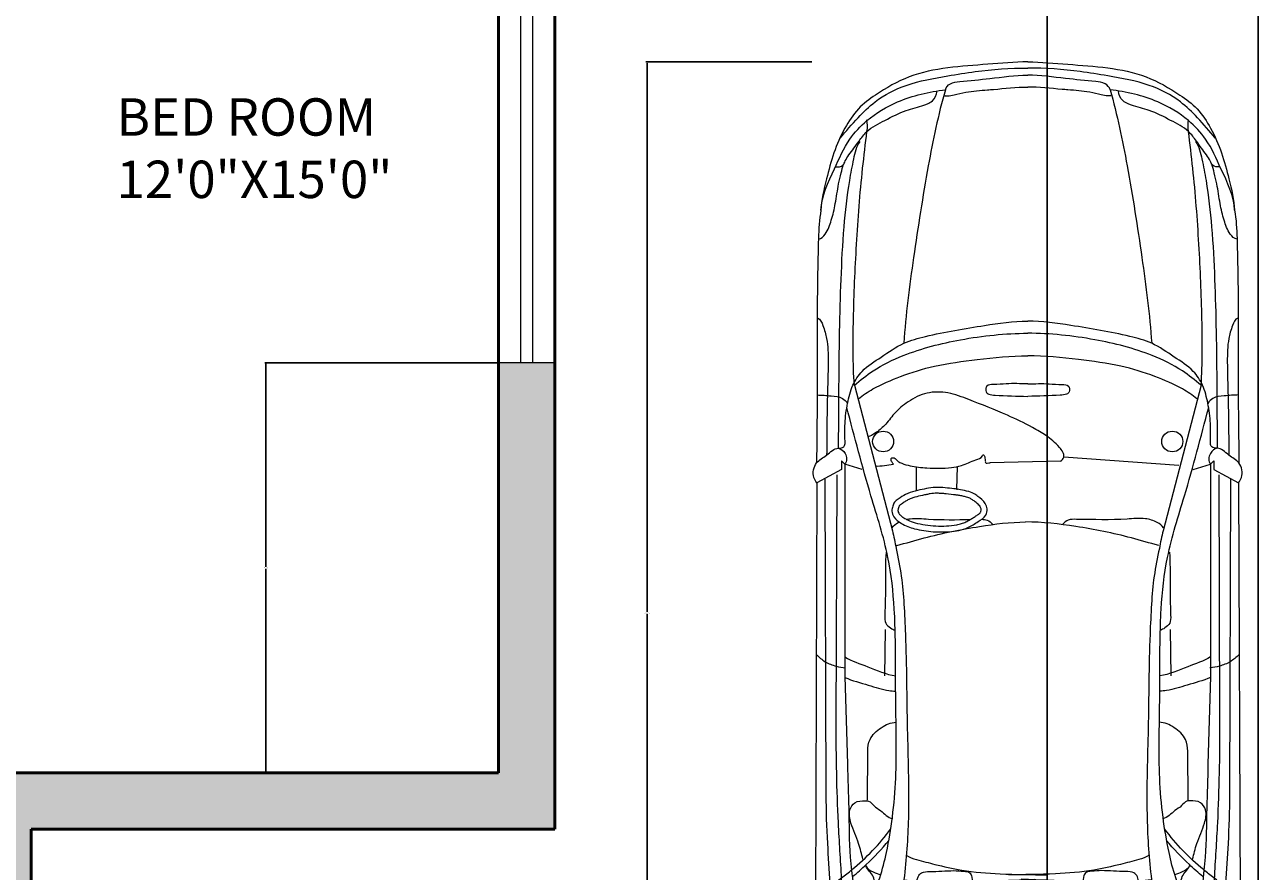
# Model space of a CAD drawing. Units: inches. Extents: x 383 to 970, y 275 to 1088.
# Tile 3 of 11: x 650 to 849, y 410 to 546. Entities that reach past the tile are written whole.
import ezdxf

# ---------------------------------------------------------------- set-up
doc = ezdxf.new("R2010")
doc.units = ezdxf.units.IN
doc.header["$MEASUREMENT"] = 0
for name, color, linetype, lineweight in [('A-ANNO-DIMS', 2, 'Continuous', 18), ('A-AREA-IDEN', 7, 'Continuous', 18), ('A-EQPM-VEHI', 8, 'Continuous', 13), ('A-GLAZ', 4, 'Continuous', 18), ('A-WALL', 7, 'Continuous', 50)]:
    doc.layers.add(name, color=color, linetype=linetype, lineweight=lineweight)
doc.layers.add('A-WALL-PATT', color=251, linetype='Continuous', lineweight=13, true_color=0x636466)
doc.styles.get("Standard").update_dxf_attribs({"font": 'arial.ttf'})
doc.dimstyles.get("Standard").update_dxf_attribs({"dimtxt": 0.18, "dimasz": 0.18, "dimexe": 0.18, "dimexo": 0.0625, "dimgap": 0.09, "dimtad": 0, "dimtih": 1, "dimtoh": 1, "dimdec": 4, "dimzin": 0, "dimdsep": 46, "dimtxsty": 'Standard', "dimcen": 0.09, "dimadec": 0, "dimazin": 0, "dimtfac": 1, "dimtdec": 4, "dimtofl": 0, "dimtmove": 0, "dimatfit": 3, "dimfxl": 1, "dimtolj": 1, "dimtzin": 0, "dimarcsym": 0})

# ---------------------------------------------------------------- blocks, each defined once
blk = doc.blocks.new('A$C242571DA')
for p, q in [((1659.9, 1632), (1714.3, 1732.5)), ((1714.3, 1732.5), (3817.1, 1739.9)), ((1699.9, 1699.4), (2984.7, 1695.8)), ((1638.3, 1618.5), (1625.1, 1632)), ((1625.1, 1632), (1659.9, 1632)), ((1638.3, 1618.5), (2503.3, 1618.5)), ((1659.9, 1548.1), (1638.3, 1618.5)), ((1681.8, 1651.6), (2695.2, 1655.3)), ((2503.3, 1618.5), (2861.6, 1607.5)), ((1317.4, 1579.7), (1909.8, 1424.9)), ((3007.2, 1526.5), (2808.1, 1525.2)), ((1644, 1489.1), (1610.4, 1020.2)), ((2311.9, 1454.3), (2500.6, 1456.9)), ((3474.6, 1401.1), (3474.6, 843)), ((4315.2, 1398), (4377.3, 1370.5)), ((1626.1, 1006.5), (1632.8, 719.7)), ((3474.6, 345.6), (3474.6, 903.8)), ((1740.2, 584.9), (1649.3, 586.9)), ((1746.1, 420.6), (1649.3, 420.6)), ((4315.2, 348.7), (4377.3, 376.3)), ((1317.4, 167), (1909.8, 321.9)), ((2311.9, 292.5), (2500.6, 289.8)), ((3007.2, 220.3), (2808.1, 221.6)), ((1659.9, 198.7), (1638.3, 128.2)), ((1638.3, 128.2), (1625.1, 114.7)), ((1625.1, 114.7), (1659.9, 114.7)), ((1638.3, 128.2), (2503.3, 128.2)), ((1659.9, 114.7), (1714.3, 14.2)), ((2503.3, 128.2), (2861.6, 139.2)), ((1681.8, 95.1), (2695.2, 91.4)), ((1699.9, 47.3), (2984.7, 51)), ((1714.3, 14.2), (3817.1, 6.9))]:
    blk.add_line(p, q)
for centre in [(1546.4, 1462.5), (1546.4, 284.2)]:
    blk.add_ellipse(centre, major_axis=(0, 42.9), ratio=0.983266, start_param=4.712389, end_param=10.995574)
for points, knots in [([(722.7, 1726.6), (720.8, 1714.9), (694.5, 1689.9), (643, 1671.8), (573.6, 1655.4), (508.5, 1647), (455.2, 1634.7), (428.7, 1627.3), (416.9, 1624.1)], [0, 0, 0, 0, 0.034703, 0.0959761, 0.1659336, 0.2471559, 0.2929944, 0.3295918, 0.3295918, 0.3295918, 0.3295918]), ([(604.6, 1715.7), (642.1, 1723.4), (788.5, 1729.2), (1039.3, 1732.2), (1344.5, 1729.9), (1542, 1733.1), (1633.8, 1733.7)], [0, 0, 0, 0, 0.114897, 0.437061, 0.754269, 1.029686, 1.029686, 1.029686, 1.029686]), ([(1043.6, 1729.2), (1048.6, 1717.9), (1080.9, 1704.2), (1138.6, 1687.6), (1237.7, 1685.6), (1394.7, 1691.3), (1521.7, 1692.4), (1601.5, 1692.7)], [0, 0, 0, 0, 0.0364992, 0.0923739, 0.1867837, 0.3273982, 0.5667068, 0.5667068, 0.5667068, 0.5667068]), ([(1356.8, 1732.2), (1357.1, 1712.8), (1360, 1678.8), (1363.9, 1630.5), (1383.3, 1613.5), (1391, 1607.2)], [0, 0, 0, 0, 1.462159, 2.651105, 3.386321, 3.386321, 3.386321, 3.386321]), ([(1714.3, 1732.5), (1707.7, 1737.6), (1683.3, 1753), (1628.7, 1741.2), (1605.6, 1691.5), (1561.7, 1652.4), (1594.1, 1610.3), (1627.9, 1608.3), (1638.3, 1618.5)], [0, 0, 0, 0, 0.024864, 0.0846267, 0.1362471, 0.1900683, 0.2245199, 0.2681841, 0.2681841, 0.2681841, 0.2681841]), ([(2414.7, 1735), (2424.9, 1723.3), (2447.2, 1698.8), (2461.2, 1657.6), (2468.1, 1629), (2468, 1616.1)], [1.808086, 1.808086, 1.808086, 1.808086, 2.918874, 4.131288, 5.10151, 5.10151, 5.10151, 5.10151]), ([(3356.5, 1739.4), (3354.9, 1719.2), (3360.8, 1678.2), (3324, 1631.5), (3255.4, 1544.3), (3187.1, 1476.2), (3125.2, 1432.2)], [0, 0, 0, 0, 0.0597371, 0.1139981, 0.1672498, 0.3938869, 0.3938869, 0.3938869, 0.3938869]), ([(3745.3, 1736.8), (3748.5, 1730.1), (3764.2, 1717.1), (3811.5, 1698.6), (3894.7, 1686.7), (4002.9, 1663.2), (4107.9, 1648.7), (4195.8, 1638.3), (4258.6, 1603.2), (4302.1, 1549.7), (4339.9, 1483.8), (4365.2, 1407.6), (4389.6, 1324.4), (4397.9, 1266.9), (4401.8, 1235.2)], [0, 0, 0, 0, 0.0219205, 0.0572122, 0.1522539, 0.2718866, 0.3894011, 0.4710097, 0.5346344, 0.5986698, 0.6733118, 0.758696, 0.8351341, 0.9293726, 0.9293726, 0.9293726, 0.9293726]), ([(3817.1, 1739.9), (3833.2, 1729.7), (3882.9, 1718.2), (3973.3, 1695.2), (4085.1, 1680.5), (4193.8, 1662.8), (4280.6, 1644.3), (4343.9, 1598.1), (4390, 1540.3), (4427.4, 1448.7), (4457.8, 1336.6), (4475.7, 1233.4), (4478.4, 1175.1), (4479.3, 1161.6)], [0, 0, 0, 0, 0.056668, 0.14946, 0.28161, 0.392935, 0.481686, 0.542967, 0.622845, 0.69797, 0.833643, 0.965665, 1.00577, 1.00577, 1.00577, 1.00577]), ([(0, 873.4), (0, 927.8), (15.6, 1088.6), (25.5, 1309.8), (120.7, 1476.4), (189.2, 1569), (273.5, 1623.1), (369.9, 1666.3), (483, 1694.7), (561.3, 1714.9), (604.6, 1715.7)], [0, 0, 0, 0, 0.16039, 0.479033, 0.632967, 0.722015, 0.817474, 0.927562, 1.03733, 1.167094, 1.167094, 1.167094, 1.167094]), ([(604.6, 1715.7), (545.5, 1714.5), (448.5, 1664.6), (320.8, 1610.6), (225.4, 1521.2), (147.3, 1390.5), (121.7, 1275.2), (113.6, 1208.7)], [0, 0, 0, 0, 0.1772572, 0.3124951, 0.4151678, 0.5597243, 0.7575412, 0.7575412, 0.7575412, 0.7575412]), ([(2984.7, 1695.8), (3051, 1695.6), (3172.1, 1691.3), (3367.4, 1677.6), (3575.2, 1664.3), (3788.2, 1643.6), (3968, 1628.1), (4103.8, 1616.8), (4203.6, 1578.1), (4271.8, 1519.5), (4300.6, 1452.1), (4341.7, 1305.3), (4361.8, 1111.2), (4367.5, 936.8), (4367.5, 873.4)], [0, 0, 0, 0, 0.198873, 0.363323, 0.587433, 0.823543, 1.004622, 1.129816, 1.230113, 1.320655, 1.388577, 1.443334, 1.771447, 1.958652, 1.958652, 1.958652, 1.958652]), ([(310.7, 1637.3), (282.5, 1613.7), (230.1, 1569.9), (148.7, 1486.2), (84.8, 1361.3), (60, 1219), (32.6, 1054.3), (25.1, 944.9), (25.1, 873.4)], [0, 0, 0, 0, 0.1095129, 0.2035347, 0.3452507, 0.5161382, 0.6275464, 0.8383798, 0.8383798, 0.8383798, 0.8383798]), ([(426.8, 1656.7), (428.5, 1646.6), (426.9, 1625), (399.8, 1616.6), (368.1, 1593.9), (328, 1564.6), (271.6, 1523.9), (237, 1451.9), (196.2, 1376.7), (183.8, 1314.9), (170, 1279.6), (157.2, 1254.2), (133.3, 1244.4), (118.6, 1242.9)], [0, 0, 0, 0, 0.0304541, 0.0502818, 0.0786089, 0.1479133, 0.1986294, 0.2831705, 0.3780326, 0.4523267, 0.4667809, 0.4902599, 0.5347198, 0.5347198, 0.5347198, 0.5347198]), ([(323.7, 1557.5), (344.8, 1571.9), (400.4, 1585.1), (516, 1606.8), (680.3, 1625.8), (885.4, 1635.7), (1116.8, 1642.2), (1346.1, 1644.2), (1504.7, 1644.7), (1574, 1645.7)], [0, 0, 0, 0, 0.076148, 0.165903, 0.355672, 0.569871, 0.782325, 1.050047, 1.257936, 1.257936, 1.257936, 1.257936]), ([(1555.2, 1617.8), (1527.7, 1617.8), (1472.5, 1620.4), (1392.7, 1608.8), (1318.5, 1591), (1249.4, 1545.5), (1201.4, 1466.7), (1142.8, 1385.7), (1104.8, 1240.4), (1076, 1072.3), (1056.4, 932.4), (1056.4, 873.4)], [0, 0, 0, 0, 0.082256, 0.165174, 0.241383, 0.30939, 0.405348, 0.511507, 0.603349, 0.843635, 1.017671, 1.017671, 1.017671, 1.017671]), ([(1574, 1645.7), (1572.9, 1638), (1574.1, 1622), (1559.9, 1618.7), (1555.2, 1617.8)], [0, 0, 0, 0, 0.02274132, 0.03717479, 0.03717479, 0.03717479, 0.03717479]), ([(2424, 1618.7), (2441.5, 1589.9), (2464.2, 1518.9), (2495.4, 1450.9), (2501.6, 1411.3)], [0, 0, 0, 0, 0.1000351, 0.2184418, 0.2184418, 0.2184418, 0.2184418]), ([(2507.7, 1618.4), (2521, 1587.7), (2536.6, 1527.1), (2559.6, 1458.5), (2563.3, 1420.6), (2563.8, 1411.4)], [0, 0, 0, 0, 2.528586, 4.711885, 5.408215, 5.408215, 5.408215, 5.408215]), ([(2695.2, 1655.3), (2829.9, 1655.3), (3041.2, 1651.4), (3351.3, 1630.7), (3527.5, 1623.2), (3626.6, 1612)], [0, 0, 0, 0, 0.4042759, 0.6333827, 0.9326252, 0.9326252, 0.9326252, 0.9326252]), ([(1317.4, 1579.7), (1227.8, 1586.1), (1036, 1584.8), (741.2, 1572.5), (486.1, 1553.3), (333.3, 1534.3), (283.3, 1528.5)], [0, 0, 0, 0, 0.269375, 0.574535, 0.885339, 1.036319, 1.036319, 1.036319, 1.036319]), ([(1317.4, 1579.7), (1296.6, 1555.5), (1247.9, 1494.4), (1177.6, 1350.5), (1124.2, 1137.4), (1105.5, 964.9), (1105.5, 873.4)], [0, 0, 0, 0, 0.0947759, 0.2311242, 0.4700259, 0.7400315, 0.7400315, 0.7400315, 0.7400315]), ([(3535.9, 1563.1), (3520.1, 1550.9), (3484.4, 1526.1), (3408.2, 1510.9), (3323.4, 1473.1), (3207.9, 1445), (3072.6, 1422.2), (2866.9, 1404.6), (2626.4, 1412.9), (2396.7, 1410.8), (2200.9, 1416.9), (2001.3, 1438.2), (1732.1, 1525.9), (1527.9, 1578.9), (1407.5, 1610.7)], [0, 0, 0, 0, 0.05975, 0.126928, 0.230034, 0.336675, 0.482225, 0.641324, 0.954906, 1.203173, 1.330375, 1.542773, 1.802261, 2.175545, 2.175545, 2.175545, 2.175545]), ([(2861.6, 1607.5), (2921.1, 1607.3), (3047.2, 1600.8), (3191.4, 1602), (3356.6, 1584.1), (3498.3, 1570.6), (3623.2, 1549.4), (3664.1, 1533.3)], [0, 0, 0, 0, 0.1783018, 0.3787173, 0.431954, 0.6762374, 0.8077184, 0.8077184, 0.8077184, 0.8077184]), ([(3248.1, 1545.2), (3226.9, 1550.4), (3176.1, 1562.1), (3113.7, 1592.9), (3052.6, 1605.3), (3010.4, 1578.8), (3010.3, 1545.3), (3010.3, 1515.9), (3033.7, 1500.1), (3052.6, 1465.2), (3078.9, 1443.5), (3084, 1424.4)], [0, 0, 0, 0, 0.0655106, 0.1550445, 0.2094604, 0.2438604, 0.287164, 0.3001388, 0.3275984, 0.3616951, 0.4200969, 0.4200969, 0.4200969, 0.4200969]), ([(3319, 1587.1), (3303.3, 1568.1), (3256.9, 1516.7), (3206.7, 1467.3), (3171.4, 1439.5)], [0, 0, 0, 0, 1.868162, 5.271297, 5.271297, 5.271297, 5.271297]), ([(3626.6, 1612), (3702.5, 1609.1), (3826.2, 1596.8), (3991.4, 1583.2), (4111.7, 1562.4), (4212.2, 1522.7), (4290.4, 1488), (4300.7, 1447.5)], [0, 0, 0, 0, 0.2277977, 0.3719478, 0.4996814, 0.5863441, 0.709615, 0.709615, 0.709615, 0.709615]), ([(1372.8, 1563.1), (1357.2, 1545), (1321.6, 1490.1), (1277, 1385.7), (1232.8, 1244.2), (1211.1, 1069.4), (1196.8, 942.4), (1196.8, 873.4)], [0, 0, 0, 0, 0.0708922, 0.1925846, 0.3348457, 0.5072814, 0.7109928, 0.7109928, 0.7109928, 0.7109928]), ([(2808.1, 1525.2), (2791.9, 1525.1), (2751.9, 1519.7), (2710.6, 1472.6), (2690, 1431.1), (2690.5, 1409.6)], [0, 0, 0, 0, 0.0486628, 0.1144515, 0.1777721, 0.1777721, 0.1777721, 0.1777721]), ([(3275.5, 1532.8), (3287.5, 1528.3), (3299.8, 1504.9), (3308.4, 1482.5), (3311.7, 1472.6)], [0, 0, 0, 0, 0.983949, 1.771691, 1.771691, 1.771691, 1.771691]), ([(3372.2, 1495.3), (3354.4, 1496.8), (3316, 1494.7), (3291.6, 1525.8), (3275.5, 1532.8)], [0, 0, 0, 0, 0.0535488, 0.1060573, 0.1060573, 0.1060573, 0.1060573]), ([(3664.1, 1533.3), (3687, 1526), (3734.8, 1502.3), (3816.7, 1444.8), (3884.1, 1342.9), (3925.1, 1239.9), (3937.3, 1177), (3940.4, 1157.6)], [0, 0, 0, 0, 0.0720749, 0.1581284, 0.2958089, 0.4262456, 0.4842292, 0.4842292, 0.4842292, 0.4842292]), ([(1898.5, 1426.2), (1889, 1420.6), (1871, 1397.2), (1856.4, 1345.2), (1867.7, 1233.5), (1864.3, 1132.3), (1863, 1038.5), (1876.9, 1022.3), (1884.5, 1015.7)], [0, 0, 0, 0, 0.842998, 2.122875, 3.997599, 9.174838, 10.012722, 10.751336, 10.751336, 10.751336, 10.751336]), ([(1909.8, 1424.9), (1933.5, 1418.7), (1995.6, 1407.6), (2094.4, 1385.8), (2211.8, 1377.1), (2419, 1366.9), (2704.7, 1366.5), (3032.7, 1354.2), (3316.2, 1371), (3558.7, 1415.9), (3789.1, 1461.7), (4028.9, 1452.9), (4196.2, 1455.2), (4292.7, 1447.9), (4300.7, 1447.5)], [0, 0, 0, 0, 0.073325, 0.188896, 0.303039, 0.425821, 0.811242, 1.159737, 1.41058, 1.660623, 1.899627, 2.11145, 2.377727, 2.401703, 2.401703, 2.401703, 2.401703]), ([(1997.2, 1450.5), (2039.7, 1454.5), (2126.7, 1451.9), (2219.8, 1454.5), (2287.1, 1456.9), (2305.7, 1434.4), (2313.2, 1419.9), (2315.8, 1413.5)], [0, 0, 0, 0, 3.267856, 6.568708, 7.399663, 8.099385, 8.621705, 8.621705, 8.621705, 8.621705]), ([(113.6, 1208.7), (215.2, 1238.6), (443.2, 1284.9), (788, 1338.7), (1029.5, 1370.7), (1146.4, 1378.6)], [0, 0, 0, 0, 0.317374, 0.69576, 1.04714, 1.04714, 1.04714, 1.04714]), ([(1969.6, 1407.3), (1960.5, 1369.8), (1927, 1259.1), (1890.9, 1078.4), (1874.3, 933), (1874.3, 864.4)], [0, 0, 0, 0, 0.1139079, 0.3411539, 0.543502, 0.543502, 0.543502, 0.543502]), ([(3231.5, 1368.3), (3240.8, 1356.2), (3253.1, 1315.7), (3271.9, 1240.7), (3297.9, 1127.9), (3310.5, 974.6), (3311.2, 858.3), (3311.6, 794.4)], [0, 0, 0, 0, 0.0451009, 0.1211996, 0.2308505, 0.385263, 0.5739042, 0.5739042, 0.5739042, 0.5739042]), ([(3294.8, 1174.5), (3294.8, 1207.4), (3299.6, 1249.5), (3298.3, 1303.9), (3326.3, 1329), (3363.9, 1320.7), (3399.3, 1329.3), (3422.1, 1315.7), (3430.7, 1297.9), (3438.7, 1234.2), (3439.6, 1174.4), (3434.7, 1112.2), (3418.9, 1102), (3395.9, 1098.6), (3362.6, 1100.9), (3331.1, 1096.6), (3298.8, 1107.6), (3297.3, 1140.3), (3294.8, 1160.9), (3294.8, 1174.5)], [0, 0, 0, 0, 0.0969044, 0.1295913, 0.1506192, 0.1985921, 0.2360698, 0.2557908, 0.2719711, 0.2929882, 0.44406, 0.4519132, 0.4720918, 0.4918599, 0.5228758, 0.5707096, 0.5892096, 0.6145759, 0.654681, 0.654681, 0.654681, 0.654681]), ([(135.5, 1213.1), (139.1, 1211.8), (138.4, 1193.3), (132.6, 1168.3), (118.8, 1111.9), (115.6, 1058.9), (109, 974.6), (102.4, 920.1), (102.4, 873.4)], [0, 0, 0, 0, 0.0114788, 0.0403472, 0.0875838, 0.1755608, 0.1991501, 0.3369659, 0.3369659, 0.3369659, 0.3369659]), ([(4401.8, 1235.2), (4411.9, 1185.3), (4421.6, 1065.8), (4424.1, 946.5), (4424.1, 878)], [0, 0, 0, 0, 0.1502861, 0.3522699, 0.3522699, 0.3522699, 0.3522699]), ([(113.6, 1208.7), (103.3, 1207), (83.6, 1187.6), (76.5, 1122.2), (68.2, 1017.3), (53.4, 925), (53.4, 873.4)], [0, 0, 0, 0, 0.0314754, 0.0702057, 0.1915753, 0.3439346, 0.3439346, 0.3439346, 0.3439346]), ([(3940.4, 1157.6), (3949.9, 1111), (3964.3, 1016.4), (3960.5, 921), (3959.8, 873.4)], [0, 0, 0, 0, 0.140379, 0.2808468, 0.2808468, 0.2808468, 0.2808468]), ([(3339.2, 1099), (3339.1, 1094.8), (3336.4, 1010.6), (3333.2, 926.3), (3330, 846.2)], [11.235438, 11.235438, 11.235438, 11.235438, 11.552536, 17.586883, 17.586883, 17.586883, 17.586883]), ([(1311.3, 873.4), (1311.2, 902.4), (1309.2, 950.9), (1315, 1002.2), (1314.2, 1039.4), (1332.1, 1044.9), (1345.7, 1044.2), (1356.8, 1028.5), (1359.2, 970.2), (1361.5, 917.6), (1362.9, 873.4)], [0, 0, 0, 0, 0.0857277, 0.1381048, 0.1641986, 0.1769751, 0.1890325, 0.2028129, 0.2286049, 0.3592554, 0.3592554, 0.3592554, 0.3592554]), ([(1626.1, 1006.5), (1623.5, 1013), (1603.1, 1029.4), (1559.1, 995), (1523, 951.9), (1480.3, 878.3), (1430.5, 774.3), (1385.5, 658.5), (1343.7, 551.3), (1343, 461.7), (1380.3, 386.9), (1428.2, 329.9), (1480.1, 294.6), (1509.8, 257.4), (1524.8, 232.6), (1528, 222.1)], [0, 0, 0, 0, 0.527288, 1.647451, 3.487558, 5.099073, 7.968657, 12.238313, 14.475187, 16.613757, 18.744202, 20.639343, 22.223389, 23.452731, 24.286529, 24.286529, 24.286529, 24.286529]), ([(3231.5, 378.5), (3240.8, 390.5), (3253.1, 431), (3271.9, 506.1), (3297.9, 618.9), (3310.5, 772.1), (3311.2, 888.4), (3311.6, 952.4)], [0, 0, 0, 0, 0.0451009, 0.1211996, 0.2308505, 0.385263, 0.5739042, 0.5739042, 0.5739042, 0.5739042]), ([(0, 873.4), (0, 819), (15.6, 658.1), (25.5, 437), (120.7, 270.3), (189.2, 177.8), (273.5, 123.7), (369.9, 80.4), (483, 52), (561.3, 31.9), (604.6, 31)], [0, 0, 0, 0, 0.16039, 0.479033, 0.632967, 0.722015, 0.817474, 0.927562, 1.03733, 1.167094, 1.167094, 1.167094, 1.167094]), ([(310.7, 109.5), (282.5, 133.1), (230.1, 176.9), (148.7, 260.5), (84.8, 385.5), (60, 527.8), (32.6, 692.4), (25.1, 801.9), (25.1, 873.4)], [0, 0, 0, 0, 0.1095129, 0.2035347, 0.3452507, 0.5161382, 0.6275464, 0.8383798, 0.8383798, 0.8383798, 0.8383798]), ([(113.6, 538.1), (103.3, 539.8), (83.6, 559.2), (76.5, 624.5), (68.2, 729.4), (53.4, 821.7), (53.4, 873.4)], [0, 0, 0, 0, 0.0314754, 0.0702057, 0.1915753, 0.3439346, 0.3439346, 0.3439346, 0.3439346]), ([(135.5, 533.6), (139.1, 534.9), (138.4, 553.4), (132.6, 578.4), (118.8, 634.9), (115.6, 687.8), (109, 772.2), (102.4, 826.7), (102.4, 873.4)], [0, 0, 0, 0, 0.0114788, 0.0403472, 0.0875838, 0.1755608, 0.1991501, 0.3369659, 0.3369659, 0.3369659, 0.3369659]), ([(1555.2, 129), (1527.7, 129), (1472.5, 126.3), (1392.7, 138), (1318.5, 155.7), (1249.4, 201.3), (1201.4, 280.1), (1142.8, 361.1), (1104.8, 506.4), (1076, 674.5), (1056.4, 814.4), (1056.4, 873.4)], [0, 0, 0, 0, 0.082256, 0.165174, 0.241383, 0.30939, 0.405348, 0.511507, 0.603349, 0.843635, 1.017671, 1.017671, 1.017671, 1.017671]), ([(1317.4, 167), (1296.6, 191.2), (1247.9, 252.4), (1177.6, 396.3), (1124.2, 609.4), (1105.5, 781.8), (1105.5, 873.4)], [0, 0, 0, 0, 0.0947759, 0.2311242, 0.4700259, 0.7400315, 0.7400315, 0.7400315, 0.7400315]), ([(1372.8, 183.6), (1357.2, 201.8), (1321.6, 256.7), (1277, 361), (1232.8, 502.6), (1211.1, 677.3), (1196.8, 804.3), (1196.8, 873.4)], [0, 0, 0, 0, 0.0708922, 0.1925846, 0.3348457, 0.5072814, 0.7109928, 0.7109928, 0.7109928, 0.7109928]), ([(1311.3, 873.4), (1311.2, 844.3), (1309.2, 795.8), (1315, 744.6), (1314.2, 707.4), (1332.1, 701.9), (1345.7, 702.6), (1356.8, 718.2), (1359.2, 776.6), (1361.5, 829.1), (1362.9, 873.4)], [0, 0, 0, 0, 0.0857277, 0.1381048, 0.1641986, 0.1769751, 0.1890325, 0.2028129, 0.2286049, 0.3592554, 0.3592554, 0.3592554, 0.3592554]), ([(1969.6, 339.5), (1960.5, 377), (1926.9, 487.6), (1892.9, 662.7), (1874.3, 801.8), (1874.3, 864.4)], [0, 0, 0, 0, 0.1139079, 0.3411539, 0.5260188, 0.5260188, 0.5260188, 0.5260188]), ([(2984.7, 51), (3051, 51.1), (3172.1, 55.5), (3367.4, 69.2), (3575.2, 82.5), (3788.2, 103.1), (3968, 118.7), (4103.8, 130), (4203.6, 168.6), (4271.8, 227.3), (4300.6, 294.7), (4341.7, 441.5), (4361.8, 635.5), (4367.5, 809.9), (4367.5, 873.4)], [0, 0, 0, 0, 0.198873, 0.363323, 0.587433, 0.823543, 1.004622, 1.129816, 1.230113, 1.320655, 1.388577, 1.443334, 1.771447, 1.958652, 1.958652, 1.958652, 1.958652]), ([(3339.2, 647.8), (3339.1, 652), (3336.4, 736.2), (3333.2, 820.5), (3330, 900.6)], [11.235438, 11.235438, 11.235438, 11.235438, 11.552536, 17.586883, 17.586883, 17.586883, 17.586883]), ([(3940.4, 589.1), (3949.9, 635.7), (3964.3, 730.4), (3960.5, 825.8), (3959.8, 873.4)], [0, 0, 0, 0, 0.140379, 0.2808468, 0.2808468, 0.2808468, 0.2808468]), ([(4401.8, 511.5), (4411.9, 561.5), (4421.6, 681), (4424.1, 800.3), (4424.1, 868.8)], [0, 0, 0, 0, 0.1502861, 0.3522699, 0.3522699, 0.3522699, 0.3522699]), ([(1639.2, 326.1), (1635.3, 323.6), (1629, 318.4), (1613.1, 314.9), (1612, 324.2), (1613.2, 330.4), (1619, 337.5), (1629, 345.7), (1637.9, 366.1), (1649, 404.8), (1656.3, 472.9), (1656.2, 543.1), (1644.6, 610.9), (1623, 651.2), (1615, 684.3), (1598.5, 691.2), (1604, 696.6), (1610.3, 699.7), (1618.8, 698.9), (1625.9, 701.3), (1638.1, 698.6), (1633, 713.4), (1632.8, 719.7)], [0, 0, 0, 0, 0.0138597, 0.0278304, 0.0329137, 0.0379971, 0.0465756, 0.0592704, 0.0762214, 0.1105991, 0.1789801, 0.2766959, 0.3173629, 0.3800771, 0.4110544, 0.4160421, 0.4210284, 0.4277212, 0.4387433, 0.4448131, 0.4508005, 0.4694463, 0.4694463, 0.4694463, 0.4694463]), ([(1740.2, 584.9), (1737.8, 571.7), (1749.5, 644.3), (1766.4, 664.5), (1792.2, 700.2), (1821.5, 709.7), (1853.1, 703.9), (1874, 668.4), (1904.5, 622.6), (1915.6, 557.2), (1915.1, 484.2), (1905.7, 417.6), (1884.9, 362.8), (1859.3, 329.1), (1831.3, 318.1), (1810.8, 322.7), (1792.2, 329.3), (1777.9, 350.3), (1753, 385.9), (1737.9, 465.8), (1728.8, 497.3), (1742.4, 597.6), (1740.2, 584.9)], [0, 0, 0, 0, 0.03969, 0.089634, 0.13125, 0.1542862, 0.1797268, 0.2207266, 0.2680991, 0.3447665, 0.4095645, 0.4843001, 0.541515, 0.5817687, 0.6060665, 0.6262474, 0.6436722, 0.6634686, 0.6988791, 0.7758465, 0.8696394, 0.907731, 0.907731, 0.907731, 0.907731]), ([(1863.4, 685.6), (1863.6, 693.5), (1865.3, 711), (1876.9, 724.5), (1884.5, 731)], [9.436432, 9.436432, 9.436432, 9.436432, 10.012722, 10.751336, 10.751336, 10.751336, 10.751336]), ([(1764.9, 587), (1765.6, 590.8), (1766.4, 595.5), (1768.5, 605.7), (1769.7, 611.3), (1773.4, 626.6), (1775.6, 633), (1779.7, 642.1), (1781.6, 644.9), (1785.7, 650.6), (1787.1, 652.5), (1793, 660.3), (1797.4, 666.2), (1804.2, 673.7), (1806.8, 676.1), (1811.1, 679.4), (1812.9, 680.5), (1816.8, 682.1), (1818.8, 682.7), (1824.4, 683.5), (1828.3, 683.2), (1832.5, 682), (1833.6, 681.5), (1836, 680.2), (1837.9, 678.7), (1842.4, 673.7), (1844.9, 670.1), (1850.3, 661.7), (1853.4, 656.6), (1859.3, 647.3), (1862.1, 642.8), (1868.3, 632.6), (1871.4, 626.9), (1876.7, 615.7), (1878.9, 609.8), (1882.8, 597.4), (1884.4, 590.8), (1888.3, 570.5), (1889.7, 556.1), (1891.2, 527.4), (1891.1, 513.1), (1888.9, 470), (1885.1, 441.2), (1874.3, 404), (1870.6, 393.8), (1863.5, 378.7), (1860.6, 373.4), (1854.4, 363.6), (1851.2, 359.2), (1845, 352.6), (1842, 350.2), (1835.8, 346.4), (1832.6, 345.3), (1828.8, 344.6), (1827.9, 344.6), (1824.6, 344.9), (1822.6, 345.2), (1817.8, 346.4), (1814.9, 347.3), (1810.9, 348.7), (1809.4, 349.4), (1808.3, 350.1), (1808.1, 350.2), (1807.3, 351), (1806.7, 351.6), (1804.7, 354), (1803.1, 356.2), (1799.6, 361.3), (1798, 363.7), (1794.9, 368.2), (1793.4, 370.4), (1789.2, 376.9), (1786.7, 381), (1782.4, 389.3), (1780.5, 393.6), (1776.9, 403), (1775.2, 408), (1770.7, 423.5), (1768.3, 434.2), (1764.9, 450.5), (1763.6, 456.4), (1761.4, 466.8), (1760.4, 471.4), (1758.1, 484.4), (1757.3, 492.6), (1757.5, 510.7), (1757.8, 516.5), (1758.6, 528.4), (1759.1, 534.3), (1761.1, 553.9), (1763.1, 570.6), (1764.4, 581.5), (1764.6, 583), (1764.7, 585), (1764.8, 585.5), (1764.8, 586.5), (1764.8, 586.7), (1764.9, 587)], [0.497033, 0.497033, 0.497033, 0.497033, 0.723444, 0.723444, 0.974636, 0.974636, 1.50964, 1.50964, 2.044645, 2.044645, 2.271061, 2.271061, 2.862376, 2.862376, 3.217654, 3.217654, 3.537253, 3.537253, 3.856852, 3.856852, 4.368613, 4.368613, 4.584627, 4.584627, 4.99269, 4.99269, 5.400753, 5.400753, 5.808816, 5.808816, 6.216879, 6.216879, 6.778716, 6.778716, 7.350371, 7.350371, 7.922025, 7.922025, 9.065335, 9.065335, 10.208644, 10.208644, 12.495263, 12.495263, 13.409896, 13.409896, 13.929088, 13.929088, 14.44828, 14.44828, 14.909885, 14.909885, 15.371489, 15.371489, 15.62524, 15.62524, 15.87899, 15.87899, 16.120875, 16.120875, 16.36276, 16.36276, 16.51635, 16.51635, 16.669941, 16.669941, 16.921521, 16.921521, 17.136676, 17.136676, 17.351831, 17.351831, 17.782142, 17.782142, 18.204974, 18.204974, 18.627807, 18.627807, 19.473473, 19.473473, 19.978923, 19.978923, 20.484372, 20.484372, 21.475119, 21.475119, 21.859144, 21.859144, 22.162884, 22.162884, 22.770362, 22.770362, 22.900493, 22.900493, 22.951221, 22.951221, 22.964298, 22.964298, 22.964298, 22.964298]), ([(1863.7, 379.4), (1862.6, 384.2), (1857.6, 413.7), (1866.5, 501.6), (1865.2, 581.4), (1864.1, 639.5)], [1.749253, 1.749253, 1.749253, 1.749253, 2.122875, 3.997599, 8.307432, 8.307432, 8.307432, 8.307432]), ([(3294.8, 572.3), (3294.8, 539.4), (3299.6, 497.2), (3298.3, 442.9), (3326.3, 417.8), (3363.9, 426), (3399.3, 417.5), (3422.1, 431), (3430.7, 448.9), (3438.7, 512.5), (3439.6, 572.4), (3434.7, 634.6), (3418.9, 644.7), (3395.9, 648.2), (3362.6, 645.9), (3331.1, 650.1), (3298.8, 639.2), (3297.3, 606.5), (3294.8, 585.9), (3294.8, 572.3)], [0, 0, 0, 0, 0.0969044, 0.1295913, 0.1506192, 0.1985921, 0.2360698, 0.2557908, 0.2719711, 0.2929882, 0.44406, 0.4519132, 0.4720918, 0.4918599, 0.5228758, 0.5707096, 0.5892096, 0.6145759, 0.654681, 0.654681, 0.654681, 0.654681]), ([(3664.1, 213.5), (3687, 220.8), (3734.8, 244.4), (3816.7, 302), (3884.1, 403.8), (3925.1, 506.9), (3937.3, 569.7), (3940.4, 589.1)], [0, 0, 0, 0, 0.0720749, 0.1581284, 0.2958089, 0.4262456, 0.4842292, 0.4842292, 0.4842292, 0.4842292]), ([(3817.1, 6.9), (3833.2, 17), (3882.9, 28.6), (3973.3, 51.5), (4085.1, 66.3), (4193.8, 84), (4280.6, 102.4), (4343.9, 148.6), (4390, 206.4), (4427.4, 298), (4457.8, 410.1), (4475.7, 513.3), (4478.4, 571.6), (4479.3, 585.2)], [0, 0, 0, 0, 0.056668, 0.14946, 0.28161, 0.392935, 0.481686, 0.542967, 0.622845, 0.69797, 0.833643, 0.965665, 1.00577, 1.00577, 1.00577, 1.00577]), ([(604.6, 31), (545.5, 32.3), (448.5, 82.2), (320.8, 136.1), (225.4, 225.5), (147.3, 356.2), (121.7, 471.5), (113.6, 538.1)], [0, 0, 0, 0, 0.1772572, 0.3124951, 0.4151678, 0.5597243, 0.7575412, 0.7575412, 0.7575412, 0.7575412]), ([(113.6, 538.1), (215.2, 508.2), (443.2, 461.9), (788, 408.1), (1029.5, 376), (1146.4, 368.2)], [0, 0, 0, 0, 0.317374, 0.69576, 1.04714, 1.04714, 1.04714, 1.04714]), ([(3745.3, 10), (3748.5, 16.7), (3764.2, 29.7), (3811.5, 48.1), (3894.7, 60.1), (4002.9, 83.6), (4107.9, 98), (4195.8, 108.4), (4258.6, 143.5), (4302.1, 197), (4339.9, 262.9), (4365.2, 339.2), (4389.6, 422.4), (4397.9, 479.8), (4401.8, 511.5)], [0, 0, 0, 0, 0.0219205, 0.0572122, 0.1522539, 0.2718866, 0.3894011, 0.4710097, 0.5346344, 0.5986698, 0.6733118, 0.758696, 0.8351341, 0.9293726, 0.9293726, 0.9293726, 0.9293726]), ([(426.8, 90), (428.5, 100.2), (426.9, 121.8), (399.8, 130.1), (368.1, 152.8), (328, 182.2), (271.6, 222.8), (237, 294.9), (196.2, 370.1), (183.8, 431.9), (170, 467.2), (157.2, 492.6), (133.3, 502.4), (118.6, 503.9)], [0, 0, 0, 0, 0.0304541, 0.0502818, 0.0786089, 0.1479133, 0.1986294, 0.2831705, 0.3780326, 0.4523267, 0.4667809, 0.4902599, 0.5347198, 0.5347198, 0.5347198, 0.5347198]), ([(1909.8, 321.9), (1933.5, 328.1), (1995.6, 339.2), (2094.4, 361), (2211.8, 369.6), (2419, 379.8), (2704.7, 380.3), (3032.7, 392.6), (3316.2, 375.8), (3558.7, 330.9), (3789.1, 285.1), (4028.9, 293.9), (4196.2, 291.5), (4292.7, 298.8), (4300.7, 299.2)], [0, 0, 0, 0, 0.073325, 0.188896, 0.303039, 0.425821, 0.811242, 1.159737, 1.41058, 1.660623, 1.899627, 2.11145, 2.377727, 2.401703, 2.401703, 2.401703, 2.401703]), ([(3535.9, 183.7), (3520.1, 195.9), (3484.4, 220.6), (3408.2, 235.8), (3323.4, 273.7), (3207.9, 301.8), (3072.6, 324.6), (2866.9, 342.1), (2626.4, 333.8), (2396.7, 335.9), (2200.9, 329.9), (2001.3, 308.6), (1732.1, 220.8), (1527.9, 167.8), (1407.5, 136)], [0, 0, 0, 0, 0.05975, 0.126928, 0.230034, 0.336675, 0.482225, 0.641324, 0.954906, 1.203173, 1.330375, 1.542773, 1.802261, 2.175545, 2.175545, 2.175545, 2.175545]), ([(1898.5, 320.6), (1889, 326.2), (1880.8, 336.8), (1874.8, 348.3), (1874, 349.7)], [0, 0, 0, 0, 0.8429982, 0.9626806, 0.9626806, 0.9626806, 0.9626806]), ([(1997.2, 296.3), (2039.7, 292.2), (2126.7, 294.9), (2219.8, 292.3), (2287.1, 289.9), (2305.7, 312.3), (2313.2, 326.9), (2315.8, 333.2)], [0, 0, 0, 0, 3.267856, 6.568708, 7.399663, 8.099385, 8.621705, 8.621705, 8.621705, 8.621705]), ([(2424, 128), (2441.5, 156.9), (2464.2, 227.8), (2495.4, 295.8), (2501.6, 335.5)], [0, 0, 0, 0, 0.1000351, 0.2184418, 0.2184418, 0.2184418, 0.2184418]), ([(2507.7, 128.3), (2521, 159.1), (2536.6, 219.7), (2559.6, 288.3), (2563.3, 326.1), (2563.8, 335.3)], [0, 0, 0, 0, 2.528586, 4.711885, 5.408215, 5.408215, 5.408215, 5.408215]), ([(2808.1, 221.6), (2791.9, 221.6), (2751.9, 227.1), (2710.6, 274.2), (2690, 315.7), (2690.5, 337.1)], [0, 0, 0, 0, 0.0486628, 0.1144515, 0.1777721, 0.1777721, 0.1777721, 0.1777721]), ([(3248.1, 201.6), (3226.9, 196.3), (3176.1, 184.7), (3113.7, 153.8), (3052.6, 141.4), (3010.4, 168), (3010.3, 201.5), (3010.3, 230.9), (3033.7, 246.6), (3052.6, 281.6), (3078.9, 303.2), (3084, 322.4)], [0, 0, 0, 0, 0.0655106, 0.1550445, 0.2094604, 0.2438604, 0.287164, 0.3001388, 0.3275984, 0.3616951, 0.4200969, 0.4200969, 0.4200969, 0.4200969]), ([(3356.5, 7.4), (3354.9, 27.5), (3360.8, 68.5), (3324, 115.2), (3255.4, 202.5), (3187.1, 270.5), (3125.2, 314.6)], [0, 0, 0, 0, 0.0597371, 0.1139981, 0.1672498, 0.3938869, 0.3938869, 0.3938869, 0.3938869]), ([(3319, 159.7), (3303.3, 178.6), (3256.9, 230), (3206.7, 279.5), (3171.4, 307.2)], [0, 0, 0, 0, 1.868162, 5.271297, 5.271297, 5.271297, 5.271297]), ([(3275.5, 214), (3287.5, 218.5), (3299.8, 241.9), (3308.4, 264.3), (3311.7, 274.2)], [0, 0, 0, 0, 0.983949, 1.771691, 1.771691, 1.771691, 1.771691]), ([(3626.6, 134.7), (3702.5, 137.7), (3826.2, 149.9), (3991.4, 163.5), (4111.7, 184.4), (4212.2, 224.1), (4290.4, 258.8), (4300.7, 299.2)], [0, 0, 0, 0, 0.2277977, 0.3719478, 0.4996814, 0.5863441, 0.709615, 0.709615, 0.709615, 0.709615]), ([(1317.4, 167), (1227.8, 160.7), (1036, 161.9), (741.2, 174.2), (486.1, 193.4), (333.3, 212.5), (283.3, 218.3)], [0, 0, 0, 0, 0.269375, 0.574535, 0.885339, 1.036319, 1.036319, 1.036319, 1.036319]), ([(2861.6, 139.2), (2921.1, 139.4), (3047.2, 146), (3191.4, 144.8), (3356.6, 162.6), (3498.3, 176.1), (3623.2, 197.4), (3664.1, 213.5)], [0, 0, 0, 0, 0.1783018, 0.3787173, 0.431954, 0.6762374, 0.8077184, 0.8077184, 0.8077184, 0.8077184]), ([(3372.2, 251.5), (3354.4, 249.9), (3316, 252), (3291.6, 220.9), (3275.5, 214)], [0, 0, 0, 0, 0.0535488, 0.1060573, 0.1060573, 0.1060573, 0.1060573]), ([(323.7, 189.2), (344.8, 174.9), (400.4, 161.7), (516, 139.9), (680.3, 121), (885.4, 111), (1116.8, 104.5), (1346.1, 102.5), (1504.7, 102), (1574, 101.1)], [0, 0, 0, 0, 0.076148, 0.165903, 0.355672, 0.569871, 0.782325, 1.050047, 1.257936, 1.257936, 1.257936, 1.257936]), ([(722.7, 20.2), (720.8, 31.8), (694.5, 56.8), (643, 75), (573.6, 91.4), (508.5, 99.8), (455.2, 112.1), (428.7, 119.5), (416.9, 122.6)], [0, 0, 0, 0, 0.034703, 0.0959761, 0.1659336, 0.2471559, 0.2929944, 0.3295918, 0.3295918, 0.3295918, 0.3295918]), ([(1356.8, 14.5), (1357.1, 33.9), (1360, 68), (1363.9, 116.3), (1383.3, 133.2), (1391, 139.5)], [0, 0, 0, 0, 1.462159, 2.651105, 3.386321, 3.386321, 3.386321, 3.386321]), ([(1574, 101.1), (1572.9, 108.7), (1574.1, 124.8), (1559.9, 128), (1555.2, 129)], [0, 0, 0, 0, 0.02274132, 0.03717479, 0.03717479, 0.03717479, 0.03717479]), ([(1714.3, 14.2), (1707.7, 9.2), (1683.3, -6.3), (1628.7, 5.5), (1605.6, 55.3), (1561.7, 94.4), (1594.1, 136.5), (1627.9, 138.5), (1638.3, 128.2)], [0, 0, 0, 0, 0.024864, 0.0846267, 0.1362471, 0.1900683, 0.2245199, 0.2681841, 0.2681841, 0.2681841, 0.2681841]), ([(2414.7, 11.8), (2424.9, 23.5), (2447.2, 48), (2461.2, 89.1), (2468.1, 117.8), (2468, 130.7)], [1.808086, 1.808086, 1.808086, 1.808086, 2.918874, 4.131288, 5.10151, 5.10151, 5.10151, 5.10151]), ([(2695.2, 91.4), (2829.9, 91.5), (3041.2, 95.4), (3351.3, 116.1), (3527.5, 123.5), (3626.6, 134.7)], [0, 0, 0, 0, 0.4042759, 0.6333827, 0.9326252, 0.9326252, 0.9326252, 0.9326252]), ([(1043.6, 17.6), (1048.6, 28.9), (1080.9, 42.6), (1138.6, 59.2), (1237.7, 61.2), (1394.7, 55.4), (1521.7, 54.3), (1601.5, 54.1)], [0, 0, 0, 0, 0.0364992, 0.0923739, 0.1867837, 0.3273982, 0.5667068, 0.5667068, 0.5667068, 0.5667068]), ([(604.6, 31), (642.1, 23.4), (788.5, 17.5), (1039.3, 14.6), (1344.5, 16.8), (1542, 13.6), (1633.8, 13.1)], [0, 0, 0, 0, 0.114897, 0.437061, 0.754269, 1.029686, 1.029686, 1.029686, 1.029686])]:
    blk.add_open_spline(points, degree=3, knots=knots)
for points in [[(283.3, 1528.5), (267.8, 1524.6), (251.4, 1527.5), (235.4, 1528.5)], [(3331.9, 1378.1), (3334.2, 1360.4), (3335.9, 1342.5), (3337.3, 1324.5)], [(4479.3, 1161.6), (4491, 1066.2), (4488, 969.5), (4488, 873.4)], [(4479.3, 585.2), (4491, 680.6), (4488, 777.3), (4488, 873.4)], [(3331.9, 368.6), (3334.2, 386.4), (3335.9, 404.3), (3337.3, 422.2)], [(1646.2, 253.1), (1647.8, 277.5), (1640, 301.6), (1639.2, 326.1)], [(283.3, 218.3), (267.8, 222.1), (251.4, 219.2), (235.4, 218.3)]]:
    blk.add_open_spline(points, degree=3)
blk = doc.blocks.new('WIN-60IN')
for p, q in [((60, 9), (0, 9)), ((60, 5.5), (0, 5.5)), ((0, 3.5), (60, 3.5)), ((0, 0), (60, 0))]:
    blk.add_line(p, q)
blk = doc.blocks.new('*D31')
at = {"layer": 'A-ANNO-DIMS', "color": 0, "lineweight": -2, "transparency": 16777216}
for p, q in [((776.51, 540.18), (749.87, 540.18)), ((750.05, 540), (750.05, 451.95)), ((750.05, 363.55), (750.05, 451.59)), ((776.51, 363.37), (749.87, 363.37))]:
    blk.add_line(p, q, dxfattribs=at)
at = {"layer": 'A-ANNO-DIMS', "color": 0, "transparency": 16777216}
for points in [[(750.02, 540), (750.08, 540), (750.05, 540.18)], [(750.02, 363.55), (750.08, 363.55), (750.05, 363.37)]]:
    blk.add_solid(points, dxfattribs=at)
at = {"layer": 'Defpoints', "color": 0, "transparency": 16777216}
for p in [(776.57, 540.18), (750.05, 363.37), (776.57, 363.37)]:
    blk.add_point(p, dxfattribs=at)
at = {"layer": 'A-ANNO-DIMS', "color": 0, "transparency": 16777216, "insert": (750.05, 451.77), "char_height": 0.18, "attachment_point": 5}
blk.add_mtext('\\A1;CAR 177', dxfattribs=at)
blk = doc.blocks.new('*D57')
at = {"layer": 'A-ANNO-DIMS', "color": 0, "lineweight": -2, "transparency": 16777216}
for p, q in [((814.24, 615.07), (814.24, 274.61)), ((848.09, 615.07), (848.09, 274.61)), ((814.42, 274.79), (830.77, 274.79)), ((847.91, 274.79), (831.56, 274.79))]:
    blk.add_line(p, q, dxfattribs=at)
at = {"layer": 'A-ANNO-DIMS', "color": 0, "transparency": 16777216}
for points in [[(814.42, 274.82), (814.42, 274.76), (814.24, 274.79)], [(847.91, 274.82), (847.91, 274.76), (848.09, 274.79)]]:
    blk.add_solid(points, dxfattribs=at)
at = {"layer": 'Defpoints', "color": 0, "transparency": 16777216}
for p in [(814.24, 615.14), (848.09, 615.14), (848.09, 274.79)]:
    blk.add_point(p, dxfattribs=at)
at = {"layer": 'A-ANNO-DIMS', "color": 0, "transparency": 16777216, "insert": (831.16, 274.79), "char_height": 0.18, "attachment_point": 5}
blk.add_mtext('\\A1;33.85', dxfattribs=at)
blk = doc.blocks.new('*D65')
at = {"layer": 'A-ANNO-DIMS', "color": 0, "lineweight": -2, "transparency": 16777216}
for p, q in [((726.18, 491.92), (688.71, 491.92)), ((688.89, 491.74), (688.89, 459.21)), ((688.89, 426.32), (688.89, 458.85)), ((726.18, 426.14), (688.71, 426.14))]:
    blk.add_line(p, q, dxfattribs=at)
at = {"layer": 'A-ANNO-DIMS', "color": 0, "transparency": 16777216}
for points in [[(688.86, 491.74), (688.92, 491.74), (688.89, 491.92)], [(688.86, 426.32), (688.92, 426.32), (688.89, 426.14)]]:
    blk.add_solid(points, dxfattribs=at)
at = {"layer": 'Defpoints', "color": 0, "transparency": 16777216}
for p in [(688.89, 491.92), (726.24, 491.92), (726.24, 426.14)]:
    blk.add_point(p, dxfattribs=at)
at = {"layer": 'A-ANNO-DIMS', "color": 0, "transparency": 16777216, "insert": (688.89, 459.03), "char_height": 0.18, "attachment_point": 5}
blk.add_mtext('\\A1;65.79', dxfattribs=at)

msp = doc.modelspace()

# ---------------------------------------------------------------- hatches: boundary and pattern name
at = {"layer": 'A-WALL-PATT'}
h = msp.add_hatch(color=256, dxfattribs=at)
h.dxf.hatch_style = 1
h.paths.add_polyline_path([(651.24, 321.1365), (651.24, 417.1365), (735.24, 417.1365), (735.24, 491.9233), (726.24, 491.9233), (726.24, 426.1365), (582.24, 426.1365), (582.24, 606.1365), (687.24, 606.1365), (687.24, 615.1365), (573.24, 615.1365), (573.24, 546.1365), (570.24, 546.1365), (570.24, 537.1365), (573.24, 537.1365), (573.24, 414.1365), (582.24, 414.1365), (582.24, 417.1365), (642.24, 417.1365), (642.24, 321.1365), (621.6203, 321.1365), (621.6203, 312.1365), (651.24, 312.1365)], flags=17)
h.paths.add_polyline_path([(597.6203, 321.1365), (582.24, 321.1365), (582.24, 390.1365), (573.24, 390.1365), (573.24, 321.1365), (570.24, 321.1365), (570.24, 312.1365), (573.24, 312.1365), (597.6203, 312.1365)], flags=16)
h.paths.add_polyline_path([(534.24, 321.1365), (500.8868, 321.1365), (500.8868, 312.1365), (534.24, 312.1365)], flags=17)
h.paths.add_polyline_path([(735.24, 606.1365), (738.24, 606.1365), (738.24, 615.1365), (723.24, 615.1365), (723.24, 606.1365), (726.24, 606.1365), (726.24, 551.9233), (735.24, 551.9233)], flags=17)
h.paths.add_polyline_path([(848.0899, 615.1365), (814.24, 615.1365), (814.24, 689.38), (805.24, 689.38), (805.24, 615.1365), (802.24, 615.1365), (802.24, 606.1365), (848.0899, 606.1365)], flags=17)
h.paths.add_polyline_path([(530.24, 615.1365), (498.24, 615.1365), (498.24, 646.5351), (489.24, 646.5351), (489.24, 615.1365), (466.771, 615.1365), (466.771, 606.1365), (521.24, 606.1365), (521.24, 603.1365), (530.24, 603.1365), (530.24, 606.1365)], flags=17)
h.paths.add_polyline_path([(498.24, 744.1365), (489.24, 744.1365), (489.24, 706.5351), (498.24, 706.5351)], flags=17)
h.paths.add_polyline_path([(715.24, 792.1365), (598.24, 792.1365), (598.24, 972.1365), (636.5058, 972.1365), (636.5058, 981.1365), (589.24, 981.1365), (589.24, 972.1365), (589.24, 792.1365), (586.24, 792.1365), (586.24, 783.1365), (589.24, 783.1365), (715.24, 783.1365)], flags=17)
h.paths.add_polyline_path([(763.24, 981.1365), (696.5058, 981.1365), (696.5058, 972.1365), (754.24, 972.1365), (754.24, 792.1365), (751.24, 792.1365), (751.24, 783.1365), (754.24, 783.1365), (764.24, 783.1365), (764.24, 792.1365), (763.24, 792.1365)], flags=17)
h.paths.add_polyline_path([(815.24, 1001.9492), (806.24, 1001.9492), (806.24, 972.1365), (818.24, 972.1365), (818.24, 981.1365), (815.24, 981.1365)], flags=17)
h.paths.add_polyline_path([(546.24, 1004.0336), (537.24, 1004.0336), (537.24, 981.1365), (534.24, 981.1365), (534.24, 972.1365), (537.24, 972.1365), (546.24, 972.1365), (546.24, 981.1365)], flags=17)
h.paths.add_polyline_path([(884.0899, 606.1365), (932.24, 606.1365), (932.24, 1050.1365), (420.24, 1050.1365), (420.24, 312.1365), (440.8868, 312.1365), (440.8868, 321.1365), (429.24, 321.1365), (429.24, 537.1365), (538.24, 537.1365), (538.24, 546.1365), (530.24, 546.1365), (530.24, 579.1365), (521.24, 579.1365), (521.24, 546.1365), (429.24, 546.1365), (429.24, 606.1365), (442.771, 606.1365), (442.771, 615.1365), (429.24, 615.1365), (429.24, 783.1365), (489.24, 783.1365), (489.24, 780.1365), (498.24, 780.1365), (498.24, 783.1365), (550.24, 783.1365), (550.24, 792.1365), (429.24, 792.1365), (429.24, 972.1365), (510.24, 972.1365), (510.24, 981.1365), (429.24, 981.1365), (429.24, 1041.1365), (537.24, 1041.1365), (537.24, 1028.0336), (546.24, 1028.0336), (546.24, 1041.1365), (806.24, 1041.1365), (806.24, 1025.9492), (815.24, 1025.9492), (815.24, 1041.1365), (923.24, 1041.1365), (923.24, 981.1365), (842.24, 981.1365), (842.24, 972.1365), (923.24, 972.1365), (923.24, 792.1365), (800.24, 792.1365), (800.24, 783.1365), (805.24, 783.1365), (805.24, 725.38), (814.24, 725.38), (814.24, 783.1365), (923.24, 783.1365), (923.24, 615.1365), (884.0899, 615.1365)])

# ---------------------------------------------------------------- linework, layer by layer
at = {"layer": 'A-GLAZ'}
msp.add_line((735.24, 491.9233), (726.24, 491.9233), dxfattribs=at)
at = {"layer": 'A-WALL'}
for p, q in [((726.24, 606.1365), (726.24, 426.1365)), ((735.24, 606.1365), (735.24, 417.1365)), ((582.24, 426.1365), (726.24, 426.1365)), ((651.24, 417.1365), (651.24, 321.1365)), ((651.24, 417.1365), (735.24, 417.1365))]:
    msp.add_line(p, q, dxfattribs=at)

# ---------------------------------------------------------------- block references
at = {"layer": 'A-EQPM-VEHI', "xscale": 0.0393700787401575, "yscale": 0.0393700787401575, "zscale": 0.0393700787401575, "rotation": 270}
msp.add_blockref('A$C242571DA', (776.7342, 540.1782), dxfattribs=at)
at = {"layer": 'A-GLAZ', "rotation": 90.00000000000003}
msp.add_blockref('WIN-60IN', (735.2405, 491.9235), dxfattribs=at)

# ---------------------------------------------------------------- texts
at = {"layer": 'A-AREA-IDEN', "insert": (664.9443, 534.3444), "char_height": 6, "attachment_point": 1}
msp.add_mtext_dynamic_manual_height_columns('BED ROOM\\P12\'0"X15\'0"', width=50.211774, gutter_width=30, heights=[0], dxfattribs=at)

# ---------------------------------------------------------------- dimensions: what is measured, and where the dimension line sits
at = {"layer": 'A-ANNO-DIMS'}
dim = msp.add_linear_dim(base=(848.0899, 274.7865), p1=(814.24, 615.1365), p2=(848.0899, 615.1365), dimstyle='Standard', override={"dimdec": 2, "dimlfac": 1, "dimrnd": 0, "dimzin": 0, "dimdsep": 46, "dimlunit": 2}, dxfattribs=at)
dim.commit()
dim.dimension.update_dxf_attribs({"geometry": '*D57', "text_midpoint": (831.165, 274.7865)})
dim = msp.add_linear_dim(base=(750.0505, 363.3653), p1=(776.5724, 540.1782), p2=(776.5724, 363.3653), angle=270, text='CAR <>', dimstyle='Standard', override={"dimdec": 0, "dimlfac": 1, "dimrnd": 0, "dimzin": 0, "dimdsep": 46, "dimlunit": 2}, dxfattribs=at)
dim.commit()
dim.dimension.update_dxf_attribs({"geometry": '*D31', "text_midpoint": (750.0505, 451.7717)})
dim = msp.add_linear_dim(base=(688.89, 491.9233), p1=(726.24, 426.1365), p2=(726.24, 491.9233), angle=90, dimstyle='Standard', override={"dimdec": 2, "dimlfac": 1, "dimrnd": 0, "dimzin": 0, "dimdsep": 46, "dimlunit": 2}, dxfattribs=at)
dim.commit()
dim.dimension.update_dxf_attribs({"geometry": '*D65', "text_midpoint": (688.89, 459.0299)})

doc.saveas('drawing.dxf')
